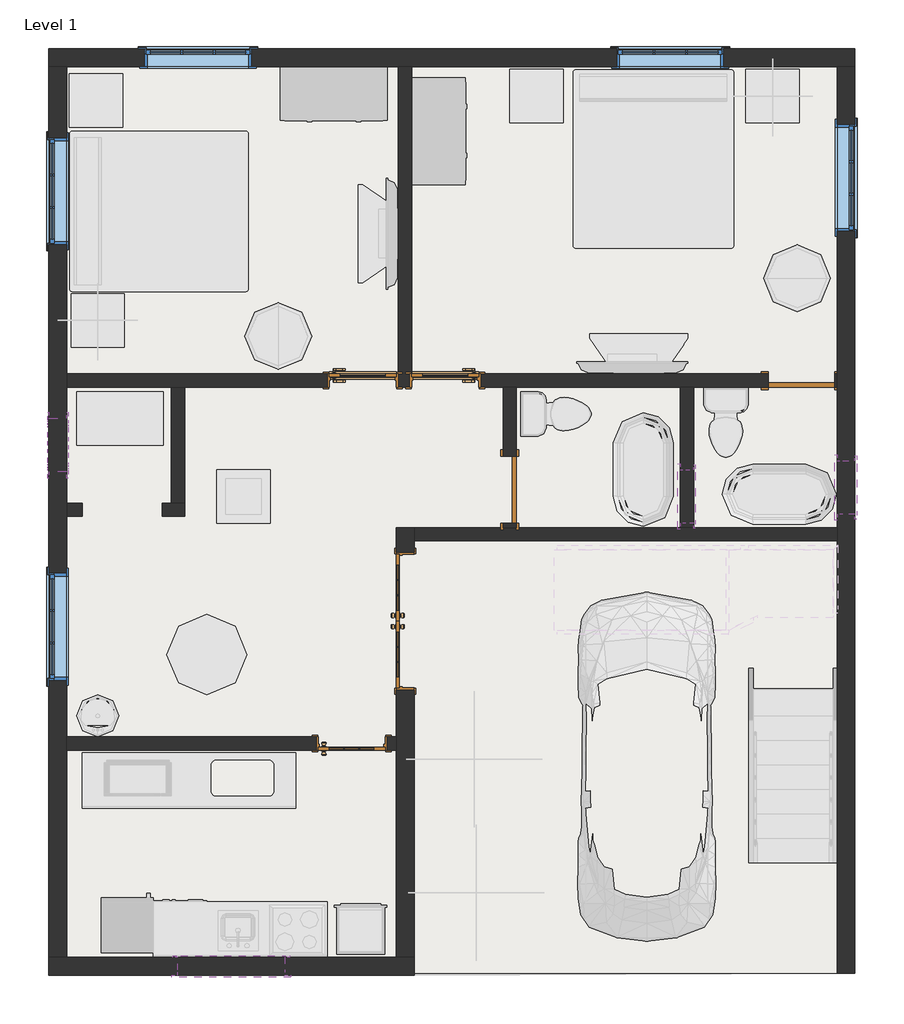
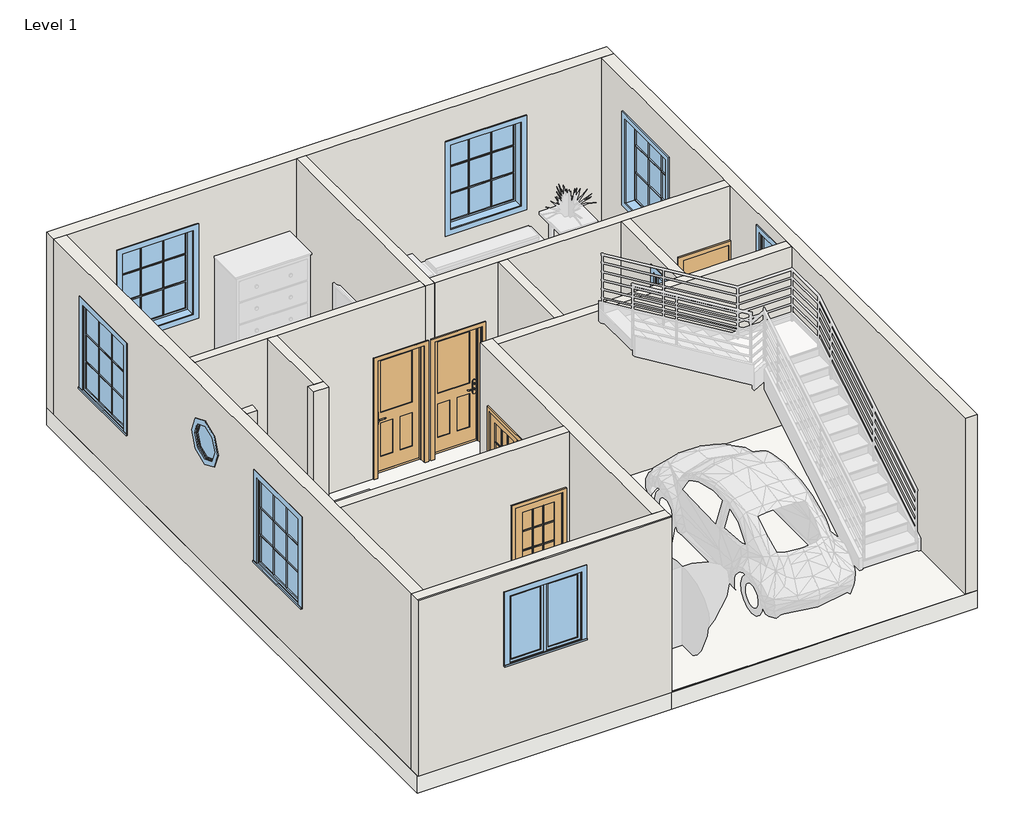
# One storey, part 1 of 5: 15 walls, 9 windows, 6 doors, 1 slab.
"""IFC4 building model written with IfcOpenShell, lengths in millimetres."""

from ifc_helpers import new_model, si_unit, frame, origin, origin_with_axes, place, context, project, spatial, polyline, circle_curve, outline, extrude, faceted_brep, transform, mapped, element, save
from ifc_brep_helpers import plane_surface, revolved_surface, advanced_brep
from components import door_cdf9d6cc, door_ce1fc124, door_9d00318c, door_a0b5ff2a, door_059fdd7e, door_255cab33, window_cfa1ffdd, window_0862ab64, window_99b8bbb7, window_e41d21a6, window_3d781103

model = new_model("IFC4")

# Units and contexts
model_context = context("Model", 3, world=origin())
ifc_project = project(units=[si_unit("LENGTHUNIT", "METRE", prefix="MILLI")], contexts=[model_context])

# Site, building, storey
site = spatial("IfcSite", under=ifc_project)
building = spatial("IfcBuilding", under=site)
storey = spatial("IfcBuildingStorey", under=building, Name="Level 1", Elevation=0.0)

# Doors
placement = place(None, origin())
door_shape = door_cdf9d6cc(model_context)
element("IfcDoor", 1, ObjectType="30\" x 80\"", at=placement, inside=storey, context=model_context, shape_type="MappedRepresentation", body=[
    mapped(door_shape, transform((-5627.3730118, 8857.4950123, 0.0), x_axis=(1.0, 0.0, 0.0), y_axis=(0.0, 1.0, 0.0), z_axis=(0.0, 0.0, 1.0))),
])
door_2_shape = door_ce1fc124(model_context)
element("IfcDoor", 2, ObjectType="30\" x 80\"", at=placement, inside=storey, context=model_context, shape_type="MappedRepresentation", body=[
    mapped(door_2_shape, transform((-6567.1730118, 8857.4950123, 0.0), x_axis=(-1.0, 0.0, 0.0), y_axis=(0.0, -1.0, 0.0), z_axis=(0.0, 0.0, 1.0))),
])
door_3_shape = door_9d00318c(model_context)
element("IfcDoor", 3, ObjectType="Door-Interior-Double-Full Glass-Wood : 60\" x 80\"", at=placement, inside=storey, context=model_context, shape_type="MappedRepresentation", body=[
    mapped(door_3_shape, transform((-6087.7480118, 6111.1200123, 0.0), x_axis=(0.0, 1.0, 0.0), y_axis=(-1.0, 0.0, 0.0), z_axis=(0.0, 0.0, 1.0))),
])
door_4_shape = door_a0b5ff2a(model_context)
element("IfcDoor", 4, ObjectType="Door-Interior-Single-Full Glass-Wood : 30\" x 80\"", at=placement, inside=storey, context=model_context, shape_type="MappedRepresentation", body=[
    mapped(door_4_shape, transform((-6694.1730118, 4710.9450123, 0.0), x_axis=(1.0, 0.0, 0.0), y_axis=(0.0, 1.0, 0.0), z_axis=(0.0, 0.0, 1.0))),
])
door_5_shape = door_059fdd7e(model_context)
element("IfcDoor", 5, ObjectType="Single-Flush : 30\" x 80\"", at=placement, inside=storey, context=model_context, shape_type="MappedRepresentation", body=[
    mapped(door_5_shape, transform((-4890.7730118, 7609.7200123, 0.0), x_axis=(0.0, -1.0, 0.0), y_axis=(1.0, 0.0, 0.0), z_axis=(0.0, 0.0, 1.0))),
])
door_6_shape = door_255cab33(model_context)
element("IfcDoor", 6, ObjectType="Single-Flush : 30\" x 80\"", at=placement, inside=storey, context=model_context, shape_type="MappedRepresentation", body=[
    mapped(door_6_shape, transform((-1563.3730118, 8854.3200123, 0.0), x_axis=(1.0, 0.0, 0.0), y_axis=(0.0, 1.0, 0.0), z_axis=(0.0, 0.0, 1.0))),
])

# Slab
element("IfcSlab", 7, ObjectType="Generic - 12\"", at=placement, inside=storey, context=model_context, shape_type="SweptSolid", body=[
    extrude(outline(polyline([(-953.7730118, 12638.9200123), (-953.7730118, 7025.5200123), (-953.7730118, 2097.9200123), (-5982.9730118, 2097.9200123), (-10148.5730118, 2097.9200123), (-10148.5730118, 12638.9200123), (-953.7730118, 12638.9200123)])), frame((0.0, 0.0, -304.8), z_axis=(0.0, 0.0, 1.0), x_axis=(1.0, 0.0, 0.0)), (0.0, 0.0, 1.0), 304.8),
])

# Walls
element("IfcWall", 8, ObjectType="Generic - 8\"", at=placement, inside=storey, context=model_context, shape_type="Brep", body=[
    faceted_brep([(-10148.5730118, 12435.7200123, 0.0), (-9945.3730118, 12435.7200123, 0.0), (-6160.7730118, 12435.7200123, 0.0), (-6008.3730118, 12435.7200123, 0.0), (-1156.9730118, 12435.7200123, 0.0), (-953.7730118, 12435.7200123, 0.0), (-953.7730118, 12435.7200123, 3048.0), (-1156.9730118, 12435.7200123, 3048.0), (-6008.3730118, 12435.7200123, 3048.0), (-6160.7730118, 12435.7200123, 3048.0), (-9945.3730118, 12435.7200123, 3048.0), (-10148.5730118, 12435.7200123, 3048.0), (-2452.3730118, 12435.7200123, 2438.4), (-2452.3730118, 12435.7200123, 914.4), (-3671.5730118, 12435.7200123, 914.4), (-3671.5730118, 12435.7200123, 2438.4), (-7837.1730118, 12435.7200123, 2438.4), (-7837.1730118, 12435.7200123, 914.4), (-9056.3730118, 12435.7200123, 914.4), (-9056.3730118, 12435.7200123, 2438.4), (-10148.5730118, 12638.9200123, 0.0), (-10148.5730118, 12638.9200123, 3048.0), (-953.7730118, 12638.9200123, 3048.0), (-953.7730118, 12638.9200123, 0.0), (-2452.3730118, 12638.9200123, 2438.4), (-3671.5730118, 12638.9200123, 2438.4), (-3671.5730118, 12638.9200123, 914.4), (-2452.3730118, 12638.9200123, 914.4), (-7837.1730118, 12638.9200123, 2438.4), (-9056.3730118, 12638.9200123, 2438.4), (-9056.3730118, 12638.9200123, 914.4), (-7837.1730118, 12638.9200123, 914.4)], [[[0, 1, 2, 3, 4, 5, 6, 7, 8, 9, 10, 11], [12, 13, 14, 15], [16, 17, 18, 19]], [[20, 21, 22, 23], [24, 25, 26, 27], [28, 29, 30, 31]], [[5, 4, 3, 2, 1, 0, 20, 23]], [[6, 5, 23, 22]], [[0, 11, 21, 20]], [[11, 10, 9, 8, 7, 6, 22, 21]], [[13, 12, 24, 27]], [[14, 13, 27, 26]], [[15, 14, 26, 25]], [[12, 15, 25, 24]], [[17, 16, 28, 31]], [[18, 17, 31, 30]], [[19, 18, 30, 29]], [[16, 19, 29, 28]]]),
])
element("IfcWall", 9, ObjectType="Generic - 8\"", at=placement, inside=storey, context=model_context, shape_type="Brep", body=[
    faceted_brep([(-1156.9730118, 12435.7200123, 0.0), (-1156.9730118, 8930.5200123, 0.0), (-1156.9730118, 8778.1200123, 0.0), (-1156.9730118, 7177.9200123, 0.0), (-1156.9730118, 7025.5200123, 0.0), (-1156.9730118, 2097.9200123, 0.0), (-1156.9730118, 2097.9200123, 3048.0), (-1156.9730118, 7025.5200123, 3048.0), (-1156.9730118, 7177.9200123, 3048.0), (-1156.9730118, 8778.1200123, 3048.0), (-1156.9730118, 8930.5200123, 3048.0), (-1156.9730118, 12435.7200123, 3048.0), (-1156.9730118, 10556.1200123, 2438.4), (-1156.9730118, 10556.1200123, 914.4), (-1156.9730118, 11775.3200123, 914.4), (-1156.9730118, 11775.3200123, 2438.4), (-1156.9730118, 7939.9200123, 2768.6), (-1156.9730118, 7330.3200123, 2768.6), (-1156.9730118, 7330.3200123, 2159.0), (-1156.9730118, 7939.9200123, 2159.0), (-953.7730118, 12435.7200123, 0.0), (-953.7730118, 12435.7200123, 3048.0), (-953.7730118, 2097.9200123, 3048.0), (-953.7730118, 2097.9200123, 0.0), (-953.7730118, 10556.1200123, 2438.4), (-953.7730118, 11775.3200123, 2438.4), (-953.7730118, 11775.3200123, 914.4), (-953.7730118, 10556.1200123, 914.4), (-953.7730118, 7939.9200123, 2768.6), (-953.7730118, 7939.9200123, 2159.0), (-953.7730118, 7330.3200123, 2159.0), (-953.7730118, 7330.3200123, 2768.6)], [[[0, 1, 2, 3, 4, 5, 6, 7, 8, 9, 10, 11], [12, 13, 14, 15], [16, 17, 18, 19]], [[20, 21, 22, 23], [24, 25, 26, 27], [28, 29, 30, 31]], [[5, 4, 3, 2, 1, 0, 20, 23]], [[6, 5, 23, 22]], [[0, 11, 21, 20]], [[11, 10, 9, 8, 7, 6, 22, 21]], [[13, 12, 24, 27]], [[14, 13, 27, 26]], [[15, 14, 26, 25]], [[12, 15, 25, 24]], [[29, 28, 16, 19]], [[30, 29, 19, 18]], [[31, 30, 18, 17]], [[28, 31, 17, 16]]]),
])
element("IfcWall", 10, ObjectType="Generic - 8\"", at=placement, inside=storey, context=model_context, shape_type="AdvancedBrep", body=[
    advanced_brep(
    [(-9945.3730118, 2275.7200123, 0.0), (-9945.3730118, 4637.9200123, 0.0), (-9945.3730118, 4790.3200123, 0.0), (-9945.3730118, 7304.9200123, 0.0), (-9945.3730118, 7457.3200123, 0.0), (-9945.3730118, 8778.1200123, 0.0), (-9945.3730118, 8930.5200123, 0.0), (-9945.3730118, 12435.7200123, 0.0), (-9945.3730118, 12435.7200123, 3048.0), (-9945.3730118, 8930.5200123, 3048.0), (-9945.3730118, 8778.1200123, 3048.0), (-9945.3730118, 7457.3200123, 3048.0), (-9945.3730118, 7304.9200123, 3048.0), (-9945.3730118, 4790.3200123, 3048.0), (-9945.3730118, 4637.9200123, 3048.0), (-9945.3730118, 2275.7200123, 3048.0), (-9945.3730118, 6657.2200123, 2438.4), (-9945.3730118, 6657.2200123, 914.4), (-9945.3730118, 5438.0200123, 914.4), (-9945.3730118, 5438.0200123, 2438.4), (-9945.3730118, 11622.9200123, 2438.4), (-9945.3730118, 11622.9200123, 914.4), (-9945.3730118, 10403.7200123, 914.4), (-9945.3730118, 10403.7200123, 2438.4), (-9945.3730118, 7812.9200123, 2133.6), (-9945.3730118, 8422.5200123, 2133.6), (-10148.5730118, 2275.7200123, 0.0), (-10148.5730118, 2275.7200123, 3048.0), (-10148.5730118, 12435.7200123, 3048.0), (-10148.5730118, 12435.7200123, 0.0), (-10148.5730118, 6657.2200123, 2438.4), (-10148.5730118, 5438.0200123, 2438.4), (-10148.5730118, 5438.0200123, 914.4), (-10148.5730118, 6657.2200123, 914.4), (-10148.5730118, 11622.9200123, 2438.4), (-10148.5730118, 10403.7200123, 2438.4), (-10148.5730118, 10403.7200123, 914.4), (-10148.5730118, 11622.9200123, 914.4), (-10148.5730118, 7812.9200123, 2133.6), (-10148.5730118, 8422.5200123, 2133.6)],
    [
        (0, 1),
        (1, 2),
        (2, 3),
        (3, 4),
        (4, 5),
        (5, 6),
        (6, 7),
        (7, 8),
        (8, 9),
        (9, 10),
        (10, 11),
        (11, 12),
        (12, 13),
        (13, 14),
        (14, 15),
        (15, 0),
        (16, 17),
        (17, 18),
        (18, 19),
        (19, 16),
        (20, 21),
        (21, 22),
        (22, 23),
        (23, 20),
        (24, 25, circle_curve(frame((-9945.3730118, 8117.7200123, 2133.6), z_axis=(-1.0, 0.0, 0.0), x_axis=(0.0, 1.0, 0.0)), 304.8)),
        (25, 24, circle_curve(frame((-9945.3730118, 8117.7200123, 2133.6), z_axis=(-1.0, 0.0, 0.0), x_axis=(0.0, 1.0, 0.0)), 304.8)),
        (26, 27),
        (27, 28),
        (28, 29),
        (29, 26),
        (30, 31),
        (31, 32),
        (32, 33),
        (33, 30),
        (34, 35),
        (35, 36),
        (36, 37),
        (37, 34),
        (38, 39, circle_curve(frame((-10148.5730118, 8117.7200123, 2133.6), z_axis=(1.0, 0.0, 0.0), x_axis=(0.0, 1.0, 0.0)), 304.8)),
        (39, 38, circle_curve(frame((-10148.5730118, 8117.7200123, 2133.6), z_axis=(1.0, 0.0, 0.0), x_axis=(0.0, 1.0, 0.0)), 304.8)),
        (0, 26),
        (29, 7),
        (28, 8),
        (15, 27),
        (16, 30),
        (33, 17),
        (32, 18),
        (31, 19),
        (20, 34),
        (37, 21),
        (36, 22),
        (35, 23),
        (38, 24),
        (25, 39),
    ],
    [
        plane_surface(frame((-9945.3730118, 2174.1200123, 0.0), z_axis=(1.0, 0.0, 0.0), x_axis=(0.0, 1.0, 0.0))),
        plane_surface(frame((-10148.5730118, 2174.1200123, 0.0), z_axis=(-1.0, 0.0, 0.0), x_axis=(0.0, -1.0, 0.0))),
        plane_surface(frame((-9945.3730118, 2174.1200123, 0.0), z_axis=(0.0, 0.0, -1.0), x_axis=(-1.0, 0.0, 0.0))),
        plane_surface(frame((-10046.9730118, 12435.7200123, 0.0), z_axis=(0.0, 1.0, 0.0), x_axis=(1.0, 0.0, 0.0))),
        plane_surface(frame((-1055.3730118, 2275.7200123, 0.0), z_axis=(0.0, -1.0, 0.0), x_axis=(-1.0, 0.0, 0.0))),
        plane_surface(frame((-10148.5730118, 12638.9200123, 3048.0), z_axis=(0.0, 0.0, 1.0), x_axis=(1.0, 0.0, 0.0))),
        plane_surface(frame((-9945.3730118, 6657.2200123, 2438.4), z_axis=(0.0, -1.0, 0.0), x_axis=(-1.0, 0.0, 0.0))),
        plane_surface(frame((-9945.3730118, 6657.2200123, 914.4), z_axis=(0.0, 0.0, 1.0), x_axis=(-1.0, 0.0, 0.0))),
        plane_surface(frame((-9945.3730118, 5438.0200123, 914.4), z_axis=(0.0, 1.0, 0.0), x_axis=(-1.0, 0.0, 0.0))),
        plane_surface(frame((-9945.3730118, 5438.0200123, 2438.4), z_axis=(0.0, 0.0, -1.0), x_axis=(-1.0, 0.0, 0.0))),
        plane_surface(frame((-9945.3730118, 11622.9200123, 2438.4), z_axis=(0.0, -1.0, 0.0), x_axis=(-1.0, 0.0, 0.0))),
        plane_surface(frame((-9945.3730118, 11622.9200123, 914.4), z_axis=(0.0, 0.0, 1.0), x_axis=(-1.0, 0.0, 0.0))),
        plane_surface(frame((-9945.3730118, 10403.7200123, 914.4), z_axis=(0.0, 1.0, 0.0), x_axis=(-1.0, 0.0, 0.0))),
        plane_surface(frame((-9945.3730118, 10403.7200123, 2438.4), z_axis=(0.0, 0.0, -1.0), x_axis=(-1.0, 0.0, 0.0))),
        revolved_surface(polyline([(-9945.3730118, 8422.5200123, 2133.6), (-10148.5730118, 8422.5200123, 2133.6)]), (-9945.3730118, 8117.7200123, 2133.6), (1.0, 0.0, 0.0)),
    ],
    [
        (0, [[1, 2, 3, 4, 5, 6, 7, 8, 9, 10, 11, 12, 13, 14, 15, 16], [17, 18, 19, 20], [21, 22, 23, 24], [25, 26]]),
        (1, [[27, 28, 29, 30], [31, 32, 33, 34], [35, 36, 37, 38], [39, 40]]),
        (2, [[-7, -6, -5, -4, -3, -2, -1, 41, -30, 42]]),
        (3, [[-8, -42, -29, 43]]),
        (4, [[-16, 44, -27, -41]]),
        (5, [[-15, -14, -13, -12, -11, -10, -9, -43, -28, -44]]),
        (6, [[-17, 45, -34, 46]]),
        (7, [[-18, -46, -33, 47]]),
        (8, [[-19, -47, -32, 48]]),
        (9, [[-20, -48, -31, -45]]),
        (10, [[-21, 49, -38, 50]]),
        (11, [[-22, -50, -37, 51]]),
        (12, [[-23, -51, -36, 52]]),
        (13, [[-24, -52, -35, -49]]),
        (14, [[-39, 53, -26, 54]]),
        (14, [[-40, -54, -25, -53]]),
    ],
),
])
element("IfcWall", 11, ObjectType="Generic - 8\"", at=placement, inside=storey, context=model_context, shape_type="Brep", body=[
    faceted_brep([(-5982.9730118, 2275.7200123, 3048.0), (-5982.9730118, 2275.7200123, 0.0), (-5982.9730118, 5323.7200123, 0.0), (-5982.9730118, 5323.7200123, 2057.4), (-5982.9730118, 6898.5200123, 2057.4), (-5982.9730118, 6898.5200123, 0.0), (-5982.9730118, 7025.5200123, 0.0), (-5982.9730118, 7177.9200123, 0.0), (-5982.9730118, 7177.9200123, 3048.0), (-5982.9730118, 7025.5200123, 3048.0), (-6186.1730118, 2275.7200123, 0.0), (-6186.1730118, 2275.7200123, 3048.0), (-6186.1730118, 4637.9200123, 3048.0), (-6186.1730118, 4790.3200123, 3048.0), (-6186.1730118, 7177.9200123, 3048.0), (-6186.1730118, 7177.9200123, 0.0), (-6186.1730118, 6898.5200123, 0.0), (-6186.1730118, 6898.5200123, 2057.4), (-6186.1730118, 5323.7200123, 2057.4), (-6186.1730118, 5323.7200123, 0.0), (-6186.1730118, 4790.3200123, 0.0), (-6186.1730118, 4637.9200123, 0.0)], [[[0, 1, 2, 3, 4, 5, 6, 7, 8, 9]], [[10, 11, 12, 13, 14, 15, 16, 17, 18, 19, 20, 21]], [[1, 10, 21, 20, 19, 2]], [[15, 7, 6, 5, 16]], [[1, 0, 11, 10]], [[8, 7, 15, 14]], [[0, 9, 8, 14, 13, 12, 11]], [[4, 17, 16, 5]], [[17, 4, 3, 18]], [[18, 3, 2, 19]]]),
])
element("IfcWall", 12, ObjectType="Generic - 8\"", at=placement, inside=storey, context=model_context, shape_type="Brep", body=[
    faceted_brep([(-5982.9730118, 2275.7200123, 0.0), (-6186.1730118, 2275.7200123, 0.0), (-9945.3730118, 2275.7200123, 0.0), (-10148.5730118, 2275.7200123, 0.0), (-10148.5730118, 2275.7200123, 3048.0), (-9945.3730118, 2275.7200123, 3048.0), (-6186.1730118, 2275.7200123, 3048.0), (-5982.9730118, 2275.7200123, 3048.0), (-8675.3730118, 2275.7200123, 2641.6), (-8675.3730118, 2275.7200123, 1422.4), (-7456.1730118, 2275.7200123, 1422.4), (-7456.1730118, 2275.7200123, 2641.6), (-5982.9730118, 2072.5200123, 0.0), (-5982.9730118, 2072.5200123, 3048.0), (-10148.5730118, 2072.5200123, 3048.0), (-10148.5730118, 2072.5200123, 0.0), (-8675.3730118, 2072.5200123, 2641.6), (-7456.1730118, 2072.5200123, 2641.6), (-7456.1730118, 2072.5200123, 1422.4), (-8675.3730118, 2072.5200123, 1422.4), (-10148.5730118, 2097.9200123, 3048.0), (-5982.9730118, 2097.9200123, 3048.0)], [[[0, 1, 2, 3, 4, 5, 6, 7], [8, 9, 10, 11]], [[12, 13, 14, 15], [16, 17, 18, 19]], [[3, 2, 1, 0, 12, 15]], [[4, 3, 15, 14, 20]], [[0, 7, 21, 13, 12]], [[20, 14, 13, 21]], [[7, 6, 5, 4, 20, 21]], [[9, 8, 16, 19]], [[10, 9, 19, 18]], [[11, 10, 18, 17]], [[8, 11, 17, 16]]]),
])
element("IfcWall", 13, ObjectType="INNER WALL", at=placement, inside=storey, context=model_context, shape_type="SweptSolid", body=[
    extrude(outline(polyline([(3048.0, -9945.3730118), (0.0, -9945.3730118), (0.0, -7100.5730118), (2057.4, -7100.5730118), (2057.4, -6287.7730118), (0.0, -6287.7730118), (0.0, -6186.1730118), (3048.0, -6186.1730118), (3048.0, -9945.3730118)])), frame((0.0, 4637.9200123, 0.0), z_axis=(0.0, 1.0, 0.0), x_axis=(0.0, 0.0, 1.0)), (0.0, 0.0, 1.0), 152.4),
])
element("IfcWall", 14, ObjectType="INNER WALL", at=placement, inside=storey, context=model_context, shape_type="Brep", body=[
    faceted_brep([(-9945.3730118, 8778.1200123, 3048.0), (-9945.3730118, 8778.1200123, 0.0), (-8751.5730118, 8778.1200123, 0.0), (-8599.1730118, 8778.1200123, 0.0), (-6973.5730118, 8778.1200123, 0.0), (-6973.5730118, 8778.1200123, 2057.4), (-6160.7730118, 8778.1200123, 2057.4), (-6160.7730118, 8778.1200123, 3048.0), (-8599.1730118, 8778.1200123, 3048.0), (-8751.5730118, 8778.1200123, 3048.0), (-9945.3730118, 8930.5200123, 0.0), (-9945.3730118, 8930.5200123, 3048.0), (-6160.7730118, 8930.5200123, 3048.0), (-6160.7730118, 8930.5200123, 2057.4), (-6973.5730118, 8930.5200123, 2057.4), (-6973.5730118, 8930.5200123, 0.0)], [[[0, 1, 2, 3, 4, 5, 6, 7, 8, 9]], [[10, 11, 12, 13, 14, 15]], [[1, 10, 15, 4, 3, 2]], [[1, 0, 11, 10]], [[12, 7, 6, 13]], [[0, 9, 8, 7, 12, 11]], [[14, 5, 4, 15]], [[5, 14, 13, 6]]]),
])
element("IfcWall", 15, ObjectType="INNER WALL", at=placement, inside=storey, context=model_context, shape_type="SweptSolid", body=[
    extrude(outline(polyline([(-9767.5730118, 7304.9200123), (-9945.3730118, 7304.9200123), (-9945.3730118, 7457.3200123), (-9767.5730118, 7457.3200123), (-9767.5730118, 7304.9200123)])), origin_with_axes(), (0.0, 0.0, 1.0), 3048.0),
])
element("IfcWall", 16, ObjectType="INNER WALL", at=placement, inside=storey, context=model_context, shape_type="SweptSolid", body=[
    extrude(outline(polyline([(-8599.1730118, 8778.1200123), (-8599.1730118, 7457.3200123), (-8751.5730118, 7457.3200123), (-8751.5730118, 8778.1200123), (-8599.1730118, 8778.1200123)])), origin_with_axes(), (0.0, 0.0, 1.0), 3048.0),
])
element("IfcWall", 17, ObjectType="INNER WALL", at=placement, inside=storey, context=model_context, shape_type="Brep", body=[
    faceted_brep([(-1156.9730118, 8778.1200123, 0.0), (-1156.9730118, 8778.1200123, 3048.0), (-2795.2730118, 8778.1200123, 3048.0), (-2947.6730118, 8778.1200123, 3048.0), (-4814.5730118, 8778.1200123, 3048.0), (-4966.9730118, 8778.1200123, 3048.0), (-6008.3730118, 8778.1200123, 3048.0), (-6008.3730118, 8778.1200123, 2057.4), (-5220.9730118, 8778.1200123, 2057.4), (-5220.9730118, 8778.1200123, 0.0), (-4966.9730118, 8778.1200123, 0.0), (-4814.5730118, 8778.1200123, 0.0), (-2947.6730118, 8778.1200123, 0.0), (-2795.2730118, 8778.1200123, 0.0), (-1944.3730118, 8778.1200123, 0.0), (-1944.3730118, 8778.1200123, 2032.0), (-1182.3730118, 8778.1200123, 2032.0), (-1182.3730118, 8778.1200123, 0.0), (-1156.9730118, 8930.5200123, 3048.0), (-1156.9730118, 8930.5200123, 0.0), (-1182.3730118, 8930.5200123, 0.0), (-1182.3730118, 8930.5200123, 2032.0), (-1944.3730118, 8930.5200123, 2032.0), (-1944.3730118, 8930.5200123, 0.0), (-5220.9730118, 8930.5200123, 0.0), (-5220.9730118, 8930.5200123, 2057.4), (-6008.3730118, 8930.5200123, 2057.4), (-6008.3730118, 8930.5200123, 3048.0)], [[[0, 1, 2, 3, 4, 5, 6, 7, 8, 9, 10, 11, 12, 13, 14, 15, 16, 17]], [[18, 19, 20, 21, 22, 23, 24, 25, 26, 27]], [[19, 0, 17, 20]], [[23, 14, 13, 12, 11, 10, 9, 24]], [[1, 0, 19, 18]], [[6, 27, 26, 7]], [[6, 5, 4, 3, 2, 1, 18, 27]], [[21, 20, 17, 16]], [[22, 21, 16, 15]], [[23, 22, 15, 14]], [[8, 25, 24, 9]], [[25, 8, 7, 26]]]),
])
element("IfcWall", 18, ObjectType="INNER WALL", at=placement, inside=storey, context=model_context, shape_type="Brep", body=[
    faceted_brep([(-1156.9730118, 7177.9200123, 0.0), (-2795.2730118, 7177.9200123, 0.0), (-2947.6730118, 7177.9200123, 0.0), (-4814.5730118, 7177.9200123, 0.0), (-4966.9730118, 7177.9200123, 0.0), (-5982.9730118, 7177.9200123, 0.0), (-5982.9730118, 7177.9200123, 3048.0), (-4966.9730118, 7177.9200123, 3048.0), (-4814.5730118, 7177.9200123, 3048.0), (-2947.6730118, 7177.9200123, 3048.0), (-2795.2730118, 7177.9200123, 3048.0), (-1156.9730118, 7177.9200123, 3048.0), (-1156.9730118, 7025.5200123, 0.0), (-1156.9730118, 7025.5200123, 3048.0), (-5982.9730118, 7025.5200123, 3048.0), (-5982.9730118, 7025.5200123, 0.0)], [[[0, 1, 2, 3, 4, 5, 6, 7, 8, 9, 10, 11]], [[12, 13, 14, 15]], [[5, 4, 3, 2, 1, 0, 12, 15]], [[0, 11, 13, 12]], [[6, 5, 15, 14]], [[11, 10, 9, 8, 7, 6, 14, 13]]]),
])
element("IfcWall", 19, ObjectType="INNER WALL", at=placement, inside=storey, context=model_context, shape_type="Brep", body=[
    faceted_brep([(-6008.3730118, 12435.7200123, 0.0), (-6008.3730118, 12435.7200123, 3048.0), (-6008.3730118, 8930.5200123, 3048.0), (-6008.3730118, 8778.1200123, 3048.0), (-6008.3730118, 8778.1200123, 2057.4), (-6008.3730118, 8930.5200123, 2057.4), (-6008.3730118, 8930.5200123, 0.0), (-6160.7730118, 12435.7200123, 0.0), (-6160.7730118, 8778.1200123, 0.0), (-6160.7730118, 8778.1200123, 2057.4), (-6160.7730118, 8778.1200123, 3048.0), (-6160.7730118, 8930.5200123, 3048.0), (-6160.7730118, 12435.7200123, 3048.0), (-6033.7730118, 8930.5200123, 0.0), (-6033.7730118, 8778.1200123, 0.0), (-6033.7730118, 8778.1200123, 2057.4), (-6033.7730118, 8930.5200123, 2057.4)], [[[0, 1, 2, 3, 4, 5, 6]], [[7, 8, 9, 10, 11, 12]], [[8, 7, 0, 6, 13, 14]], [[1, 0, 7, 12]], [[10, 9, 8, 14, 15, 4, 3]], [[3, 2, 1, 12, 11, 10]], [[16, 13, 6, 5]], [[15, 16, 5, 4]], [[13, 16, 15, 14]]]),
])
element("IfcWall", 20, ObjectType="INNER WALL", at=placement, inside=storey, context=model_context, shape_type="SweptSolid", body=[
    extrude(outline(polyline([(8778.1200123, 0.0), (7177.9200123, 0.0), (7177.9200123, 3048.0), (8778.1200123, 3048.0), (8778.1200123, 0.0)]), holes=[polyline([(7838.3200123, 2768.6), (7228.7200123, 2768.6), (7228.7200123, 2159.0), (7838.3200123, 2159.0), (7838.3200123, 2768.6)])]), frame((-2947.6730118, 0.0, 0.0), z_axis=(1.0, 0.0, 0.0), x_axis=(0.0, 1.0, 0.0)), (0.0, 0.0, 1.0), 152.4),
])
element("IfcWall", 21, ObjectType="INNER WALL", at=placement, inside=storey, context=model_context, shape_type="SweptSolid", body=[
    extrude(outline(polyline([(7228.7200123, 2032.0), (7228.7200123, 0.0), (7177.9200123, 0.0), (7177.9200123, 3048.0), (8778.1200123, 3048.0), (8778.1200123, 0.0), (7990.7200123, 0.0), (7990.7200123, 2032.0), (7228.7200123, 2032.0)])), frame((-4966.9730118, 0.0, 0.0), z_axis=(1.0, 0.0, 0.0), x_axis=(0.0, 1.0, 0.0)), (0.0, 0.0, 1.0), 152.4),
])
element("IfcWall", 22, ObjectType="INNER WALL", at=placement, inside=storey, context=model_context, shape_type="Brep", body=[
    faceted_brep([(-8853.1730118, 7304.9200123, 0.0), (-8599.1730118, 7304.9200123, 0.0), (-8599.1730118, 7304.9200123, 3048.0), (-8853.1730118, 7304.9200123, 3048.0), (-8853.1730118, 7457.3200123, 0.0), (-8853.1730118, 7457.3200123, 3048.0), (-8751.5730118, 7457.3200123, 3048.0), (-8599.1730118, 7457.3200123, 3048.0), (-8599.1730118, 7457.3200123, 0.0), (-8751.5730118, 7457.3200123, 0.0)], [[[0, 1, 2, 3]], [[4, 5, 6, 7, 8, 9]], [[1, 0, 4, 9, 8]], [[0, 3, 5, 4]], [[2, 1, 8, 7]], [[3, 2, 7, 6, 5]]]),
])

# Windows
window_shape = window_cfa1ffdd(model_context)
element("IfcWindow", 23, ObjectType="Casement 3x3 with Trim : 48\" x 60\"", at=placement, inside=storey, context=model_context, shape_type="MappedRepresentation", body=[
    mapped(window_shape, transform((-10046.9730118, 6047.6200123, 304.8), x_axis=(0.0, 1.0, 0.0), y_axis=(-1.0, 0.0, 0.0), z_axis=(0.0, 0.0, 1.0))),
])
element("IfcWindow", 24, ObjectType="Casement 3x3 with Trim : 48\" x 60\"", at=placement, inside=storey, context=model_context, shape_type="MappedRepresentation", body=[
    mapped(window_shape, transform((-10046.9730118, 11013.3200123, 304.8), x_axis=(0.0, 1.0, 0.0), y_axis=(-1.0, 0.0, 0.0), z_axis=(0.0, 0.0, 1.0))),
])
element("IfcWindow", 25, ObjectType="Casement 3x3 with Trim : 48\" x 60\"", at=placement, inside=storey, context=model_context, shape_type="MappedRepresentation", body=[
    mapped(window_shape, transform((-3061.9730118, 12537.3200123, 304.8), x_axis=(1.0, 0.0, 0.0), y_axis=(0.0, 1.0, 0.0), z_axis=(0.0, 0.0, 1.0))),
])
element("IfcWindow", 26, ObjectType="Casement 3x3 with Trim : 48\" x 60\"", at=placement, inside=storey, context=model_context, shape_type="MappedRepresentation", body=[
    mapped(window_shape, transform((-1055.3730118, 11165.7200123, 304.8), x_axis=(0.0, -1.0, 0.0), y_axis=(1.0, 0.0, 0.0), z_axis=(0.0, 0.0, 1.0))),
])
element("IfcWindow", 27, ObjectType="Casement 3x3 with Trim : 48\" x 60\"", at=placement, inside=storey, context=model_context, shape_type="MappedRepresentation", body=[
    mapped(window_shape, transform((-8446.7730118, 12537.3200123, 304.8), x_axis=(1.0, 0.0, 0.0), y_axis=(0.0, 1.0, 0.0), z_axis=(0.0, 0.0, 1.0))),
])
window_2_shape = window_0862ab64(model_context)
element("IfcWindow", 28, ObjectType="Casement Dbl with Trim : 48\" x 48\"", at=placement, inside=storey, context=model_context, shape_type="MappedRepresentation", body=[
    mapped(window_2_shape, transform((-8065.7730118, 2193.1700123, 508.0), x_axis=(-1.0, 0.0, 0.0), y_axis=(0.0, -1.0, 0.0), z_axis=(0.0, 0.0, 1.0))),
])
window_3_shape = window_99b8bbb7(model_context)
element("IfcWindow", 29, ObjectType="Round with Trim : 24\" Diameter", at=placement, inside=storey, context=model_context, shape_type="MappedRepresentation", body=[
    mapped(window_3_shape, transform((-10046.9730118, 8270.1200123, 914.4), x_axis=(0.0, 1.0, 0.0), y_axis=(-1.0, 0.0, 0.0), z_axis=(0.0, 0.0, 1.0))),
])
window_4_shape = window_e41d21a6(model_context)
element("IfcWindow", 30, ObjectType="Transom with Trim : 24\" x 24\"", at=placement, inside=storey, context=model_context, shape_type="MappedRepresentation", body=[
    mapped(window_4_shape, transform((-1055.3730118, 7673.2200123, 0.0), x_axis=(0.0, 1.0, 0.0), y_axis=(-1.0, 0.0, 0.0), z_axis=(0.0, 0.0, 1.0))),
])
window_5_shape = window_3d781103(model_context)
element("IfcWindow", 31, ObjectType="Transom with Trim : 24\" x 24\"", at=placement, inside=storey, context=model_context, shape_type="MappedRepresentation", body=[
    mapped(window_5_shape, transform((-2871.4730118, 7571.6200123, 0.0), x_axis=(0.0, 1.0, 0.0), y_axis=(-1.0, 0.0, 0.0), z_axis=(0.0, 0.0, 1.0))),
])

save(model, "model.ifc")

# Revit data of these elements
# Type "30\" x 80\""
#   Type Mark = "9"
#   Assembly Code = "B2030100"
#   Analytic Construction = "French door, wood frame with single glass"
#   Top Rail = 0' - 4 3/4"
#   Threshold Offset [instance default] = 0' - 0 1/2"
#   Thickness = 0' - 1 3/8"
#   Thermal Resistance (R) = 1.0696 (h·ft²·°F)/BTU
#   Swing Angle [instance default] = 90.00°
#   Stiles = 0' - 4 3/4"
#   Rough Width = 2' - 8"
#   Rough Height = 6' - 9"
#   Lock Rail = 0' - 7 1/8"
#   Height = 6' - 8"
#   Width = 2' - 6"
#   Heat Transfer Coefficient (U) = 0.9350 BTU/(h·ft²·°F)
#   Door Offset [instance default] = 0' - 0"
#   Bottom Rail = 0' - 9 1/2"
#   Threshold [instance default] = yes
#   Function = 1
#   Exterior Trim [instance default] = yes
#   Trim Material = Cherry
#   Threshold Material = Cherry
#   Panel Material = Cherry
#   Glazing = Glass
#   Frame Material = Cherry
#   Door Handle Material = Aluminum
#   Visual Light Transmittance = 0
#   Solar Heat Gain Coefficient = 0
#   Wall Closure = (empty or 0)
#   Construction Type = (empty or 0)
# Type "Door-Interior-Double-Full Glass-Wood : 60\" x 80\""
#   Type Mark = "8"
#   Assembly Code = "C1020300"
#   Analytic Construction = "French door, wood frame with single glass"
#   Top Rail = 0' - 4 11/16"
#   Thickness = 0' - 1 3/8"
#   Thermal Resistance (R) = 1.0696 (h·ft²·°F)/BTU
#   Swing Angle [instance default] = 90.00°
#   Stiles = 0' - 4 3/4"
#   Rough Width = 5' - 2"
#   Rough Height = 6' - 9"
#   Panel Width = 2' - 6"
#   Height = 6' - 8"
#   Width = 5' - 0"
#   Heat Transfer Coefficient (U) = 0.9350 BTU/(h·ft²·°F)
#   Bottom Rail = 0' - 9 1/8"
#   Show Grill [instance default] = yes
#   Trim Material = Cherry
#   Panel Material = Cherry
#   Frame Material = Cherry
#   Door Handle Material = Aluminum
#   Visual Light Transmittance = 0
#   Solar Heat Gain Coefficient = 0
#   Wall Closure = (empty or 0)
#   Function = (empty or 0)
# Type "Door-Interior-Single-Full Glass-Wood : 30\" x 80\""
#   Type Mark = "10"
#   Assembly Code = "C1020300"
#   Analytic Construction = "Wood frame with single clear glass"
#   Top Rail = 0' - 4 11/16"
#   Thickness = 0' - 1 3/8"
#   Thermal Resistance (R) = 1.0102 (h·ft²·°F)/BTU
#   Swing Angle [instance default] = 90.00°
#   Stiles = 0' - 4 3/4"
#   Rough Width = 2' - 8"
#   Rough Height = 6' - 9"
#   Height = 6' - 8"
#   Width = 2' - 6"
#   Heat Transfer Coefficient (U) = 0.9900 BTU/(h·ft²·°F)
#   Bottom Rail = 0' - 9 1/8"
#   Show Grill [instance default] = yes
#   Trim Material = Cherry
#   Panel Material = Cherry
#   Frame Material = Cherry
#   Door Handle Material = Aluminum
#   Visual Light Transmittance = 0
#   Solar Heat Gain Coefficient = 0
#   Wall Closure = (empty or 0)
#   Function = (empty or 0)
# Type "Single-Flush : 30\" x 80\""
#   Type Mark = "5"
#   Construction Type Id = "MDOOR"
#   Assembly Code = "C1020"
#   Analytic Construction = "Metal"
#   Thickness = 0' - 2"
#   Heat Transfer Coefficient (U) = 0.651978 BTU/(h·ft²·°F)
#   Height = 6' - 8"
#   Trim Projection Ext = 0' - 1"
#   Trim Projection Int = 0' - 1"
#   Trim Width = 0' - 3"
#   Width = 2' - 6"
#   Define Thermal Properties by = 1
#   Door Material = Door - Panel
#   Frame Material = Door - Frame
#   Visual Light Transmittance = 0
#   Solar Heat Gain Coefficient = 0
#   Function = (empty or 0)
#   Wall Closure = (empty or 0)
# Type "Generic - 12\""
#   Assembly Code = "B1010"
#   Function = 0
#   Layers, outside or top first: 1' - 0" no material (function 1)
# Type "Generic - 8\""
#   Assembly Code = "B2010"
#   Layers, outside or top first: 0' - 8" "Asphalt Shingle" (function 1)
# Type "INNER WALL"
#   Assembly Code = "B2010"
#   Layers, outside or top first: 0' - 6" "Asphalt Shingle" (function 1)
# Type "Casement 3x3 with Trim : 48\" x 60\""
#   Type Mark = "11"
#   Construction Type Id = "GSP4R"
#   Assembly Code = "B2020100"
#   Analytic Construction = "1/8 in Pilkington single glazing"
#   Visual Light Transmittance = 0.9
#   Solar Heat Gain Coefficient = 0.78
#   Heat Transfer Coefficient (U) = 0.6496 BTU/(h·ft²·°F)
#   Height = 5' - 0"
#   Default Sill Height = 2' - 0"
#   Trim Projection - Ext. = 0' - 0 1/2"
#   Trim Projection - Int. = 0' - 0 3/4"
#   Trim Width - Exterior = 0' - 3 1/2"
#   Trim Width - Interior = 0' - 3 1/2"
#   Width = 4' - 0"
#   Window Inset = 0' - 0 3/4"
#   Define Thermal Properties by = 1
#   Glass Pane Material = Glass
#   Sash Material = Sash
#   Trim Exterior Material = Trim
#   Trim Interior Material = Trim
#   Wall Closure = (empty or 0)
# Type "Casement Dbl with Trim : 48\" x 48\""
#   Type Mark = "13"
#   Construction Type Id = "GSP4R"
#   Assembly Code = "B2020100"
#   Analytic Construction = "1/8 in Pilkington single glazing"
#   Visual Light Transmittance = 0.9
#   Solar Heat Gain Coefficient = 0.78
#   Heat Transfer Coefficient (U) = 0.6496 BTU/(h·ft²·°F)
#   Height = 4' - 0"
#   Default Sill Height = 3' - 0"
#   Trim Projection - Ext. = 0' - 0 1/2"
#   Trim Projection - Int. = 0' - 0 3/4"
#   Trim Width - Exterior = 0' - 3 1/2"
#   Trim Width - Interior = 0' - 3 1/2"
#   Width = 4' - 0"
#   Window Inset = 0' - 0 3/4"
#   Define Thermal Properties by = 1
#   Glass Pane Material = Glass
#   Sash Material = Sash
#   Trim Exterior Material = Trim
#   Trim Interior Material = Trim
#   Wall Closure = (empty or 0)
# Type "Round with Trim : 24\" Diameter"
#   Type Mark = "28"
#   Construction Type Id = "GSP4R"
#   Assembly Code = "B2020100"
#   Analytic Construction = "1/8 in Pilkington single glazing"
#   Visual Light Transmittance = 0.9
#   Solar Heat Gain Coefficient = 0.78
#   Heat Transfer Coefficient (U) = 0.6496 BTU/(h·ft²·°F)
#   Default Sill Height = 3' - 0"
#   Trim Projection - Ext. = 0' - 0 1/2"
#   Trim Projection - Int. = 0' - 0 3/4"
#   Trim Width - Exterior = 0' - 3 1/2"
#   Trim Width - Interior = 0' - 3 1/2"
#   Width = 2' - 0"
#   Define Thermal Properties by = 1
#   Glass Pane Material = Glass
#   Sash Material = Sash
#   Trim Exterior Material = Trim
#   Trim Interior Material = Trim
#   Wall Closure = (empty or 0)
# Type "Transom with Trim : 24\" x 24\""
#   Type Mark = "16"
#   Construction Type Id = "GSP4R"
#   Assembly Code = "B2020100"
#   Analytic Construction = "1/8 in Pilkington single glazing"
#   Visual Light Transmittance = 0.9
#   Solar Heat Gain Coefficient = 0.78
#   Heat Transfer Coefficient (U) = 0.6496 BTU/(h·ft²·°F)
#   Height = 2' - 0"
#   Default Sill Height = 7' - 1"
#   Trim Projection - Ext. = 0' - 0 1/2"
#   Trim Projection - Int. = 0' - 0 3/4"
#   Trim Width - Exterior = 0' - 3 1/2"
#   Trim Width - Interior = 0' - 3 1/2"
#   Width = 2' - 0"
#   Window Inset = 0' - 0 3/4"
#   Define Thermal Properties by = 1
#   Glass Pane Material = Glass
#   Sash Material = Sash
#   Trim Exterior Material = Trim
#   Trim Interior Material = Trim
#   Wall Closure = (empty or 0)
# Elements 1, 2 (IfcDoor, "30\" x 80\"")
#   Threshold Offset = 0' - 0 1/2"
#   Swing Angle = 90.00°
#   Door Offset = 0' - 0"
#   Threshold = yes
#   Exterior Trim = yes
#   Phase Created = New Construction
#   Materials on its faces: "Cherry", "Aluminum", "Glass"
# Element 3 (IfcDoor, "Door-Interior-Double-Full Glass-Wood : 60\" x 80\"")
#   Swing Angle = 90.00°
#   Show Grill = yes
#   Phase Created = New Construction
#   Materials on its faces: "Cherry", "Aluminum", "Glass"
# Element 4 (IfcDoor, "Door-Interior-Single-Full Glass-Wood : 30\" x 80\"")
#   Swing Angle = 90.00°
#   Show Grill = yes
#   Phase Created = New Construction
#   Materials on its faces: "Cherry", "Aluminum", "Glass"
# Elements 5, 6 (IfcDoor, "Single-Flush : 30\" x 80\"")
#   Phase Created = New Construction
#   Materials on its faces: "Door - Frame", "Door - Panel"
# Element 7 (IfcSlab, "Generic - 12\"")
#   Height Offset From Level = 0' - 0"
#   Phase Created = New Construction
#   Materials on its faces: "Default Floor"
# Elements 8, 9, 10, 11, 12 (IfcWall, "Generic - 8\"")
#   Top Offset = 0' - 0"
#   Base Offset = 0' - 0"
#   Unconnected Height = 10' - 0"
#   wall height = 10' - 0"
#   Phase Created = New Construction
#   Base Constraint = Level 1
#   Materials on its faces: "Asphalt Shingle"
# Elements 13, 14, 15, 16, 17, 18, 19, 20, 21, 22 (IfcWall, "INNER WALL")
#   Top Offset = 0' - 0"
#   Base Offset = 0' - 0"
#   Unconnected Height = 10' - 0"
#   wall height = 10' - 0"
#   Phase Created = New Construction
#   Base Constraint = Level 1
#   Materials on its faces: "Asphalt Shingle"
# Element 23 (IfcWindow, "Casement 3x3 with Trim : 48\" x 60\"")
#   Mark = "1"
#   Phase Created = New Construction
#   Materials on its faces: "Sash", "Glass", "Trim"
# Element 24 (IfcWindow, "Casement 3x3 with Trim : 48\" x 60\"")
#   Mark = "2"
#   Phase Created = New Construction
#   Materials on its faces: "Sash", "Glass", "Trim"
# Element 25 (IfcWindow, "Casement 3x3 with Trim : 48\" x 60\"")
#   Mark = "3"
#   Phase Created = New Construction
#   Materials on its faces: "Sash", "Glass", "Trim"
# Element 26 (IfcWindow, "Casement 3x3 with Trim : 48\" x 60\"")
#   Mark = "4"
#   Phase Created = New Construction
#   Materials on its faces: "Sash", "Glass", "Trim"
# Element 27 (IfcWindow, "Casement 3x3 with Trim : 48\" x 60\"")
#   Mark = "5"
#   Phase Created = New Construction
#   Materials on its faces: "Sash", "Glass", "Trim"
# Element 28 (IfcWindow, "Casement Dbl with Trim : 48\" x 48\"")
#   Mark = "6"
#   Phase Created = New Construction
#   Materials on its faces: "Sash", "Trim", "Glass"
# Element 29 (IfcWindow, "Round with Trim : 24\" Diameter")
#   Mark = "9"
#   Phase Created = New Construction
#   Materials on its faces: "Trim", "Sash", "Glass"
# Element 30 (IfcWindow, "Transom with Trim : 24\" x 24\"")
#   Mark = "7"
#   Phase Created = New Construction
#   Materials on its faces: "Sash", "Trim", "Glass"
# Element 31 (IfcWindow, "Transom with Trim : 24\" x 24\"")
#   Mark = "8"
#   Phase Created = New Construction
#   Materials on its faces: "Sash", "Trim", "Glass"
# Materials
#   "Cherry": class "Wood", colour RGB 226 177 128, transparency 0, Description = "Prunus Serotina", Cost = 0
#   "Glass": class "Glass", colour RGB 0 128 192, transparency 0.75, Description = "Soda Lime Glass", Cost = 0
#   "Aluminum": class "Metal", colour RGB 247 247 247, transparency 0, Description = "Aluminum 6061", Cost = 0
#   "Door - Panel": class "Wood", colour RGB 210 159 95, transparency 0
#   "Door - Frame": colour RGB 118 70 51, transparency 0
#   "Asphalt Shingle": class "Generic", colour RGB 155 155 155, transparency 0, Description = "Asphalt roofing shingle", Cost = 0
#   "Sash": class "Wood", colour RGB 224 178 126, transparency 0
#   "Trim": class "Wood", colour RGB 224 178 126, transparency 0
#   "Default Floor": colour RGB 128 128 128, transparency 0
# Room at (-8107.366, 10770.472) mm, phase "New Construction", upper level "Level 1", upper offset 10' - 0", lower offset 0' - 0"
#   Number = "1"
#   Name = "BEDROOM"
# Room at (-3334.204, 10770.472) mm, phase "New Construction", upper level "Level 1", upper offset 10' - 0", lower offset 0' - 0"
#   Number = "2"
#   Name = "BEDROOM"
# Room at (-9257.228, 7864.146) mm, phase "New Construction", upper level "Level 1", upper offset 10' - 0", lower offset 0' - 0"
#   Number = "3"
# Room at (-7428.428, 7308.812) mm, phase "New Construction", upper level "Level 1", upper offset 10' - 0", lower offset 0' - 0"
#   Number = "4"
#   Name = "HALL"
# Room at (-3926.02, 7864.146) mm, phase "New Construction", upper level "Level 1", upper offset 10' - 0", lower offset 0' - 0"
#   Number = "5"
#   Name = "TOILET"
# Room at (-1863.35, 7864.146) mm, phase "New Construction", upper level "Level 1", upper offset 10' - 0", lower offset 0' - 0"
#   Number = "6"
#   Name = "TOILET"
# Room at (-3100.952, 3834.006) mm, phase "New Construction", upper level "Level 1", upper offset 10' - 0", lower offset 0' - 0"
#   Number = "7"
#   Name = "PARKING"
# Room at (-7987.893, 3532.539) mm, phase "New Construction", upper level "Level 1", upper offset 10' - 0", lower offset 0' - 0"
#   Number = "8"
#   Name = "KITCHEN"
